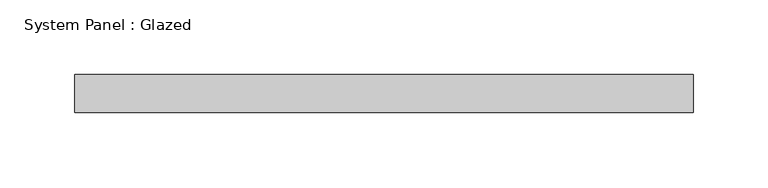
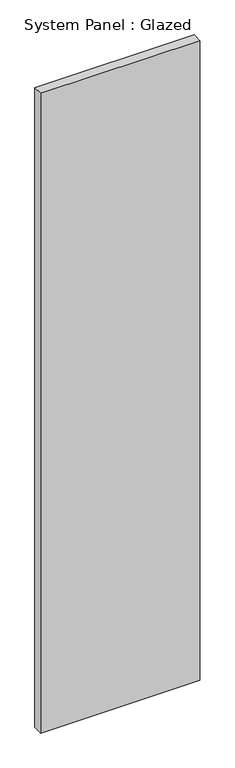
"""IFC4 building model written with IfcOpenShell, lengths in millimetres: plate geometry, System Panel : Glazed."""

from ifc_helpers import new_model, si_unit, origin, origin_with_axes, place, context, project, spatial, polyline, outline, extrude, source, transform, mapped, element, save


def system_panel_glazed_e2ad0beb(model_context):
    return source(origin(), model_context, "Body", "SweptSolid", [
        extrude(outline(polyline([(206.375, 19.05), (-206.375, 19.05), (-206.375, 44.45), (206.375, 44.45), (206.375, 19.05)])), origin_with_axes(), (0.0, 0.0, 1.0), 1752.6),
    ])


if __name__ == "__main__":
    model = new_model("IFC4")
    model_context = context("Model", 3, world=origin())
    ifc_project = project(units=[si_unit("LENGTHUNIT", "METRE", prefix="MILLI")], contexts=[model_context])
    site = spatial("IfcSite", under=ifc_project)
    building = spatial("IfcBuilding", under=site)
    placement = place(None, origin())
    system_panel_glazed_shape = system_panel_glazed_e2ad0beb(model_context)
    element("IfcPlate", 1, ObjectType="System Panel : Glazed", at=placement, inside=building, context=model_context, shape_type="MappedRepresentation", body=[
        mapped(system_panel_glazed_shape, transform((0.0, 0.0, 0.0), x_axis=(1.0, 0.0, 0.0), y_axis=(0.0, 1.0, 0.0), z_axis=(0.0, 0.0, 1.0))),
    ])
    save(model, "model.ifc")

# Revit data of these elements
# Type "System Panel : Glazed"
#   Construction Type Id = "GSP4R"
#   Analytic Construction = "1/8 in Pilkington single glazing"
#   Visual Light Transmittance = 0.9
#   Solar Heat Gain Coefficient = 0.86
#   Heat Transfer Coefficient (U) = 1.18115 BTU/(h·ft²·°F)
#   Define Thermal Properties by = 1
# Element 1 (IfcPlate, "System Panel : Glazed")
#   Materials on its faces: "Glass"
# Materials
#   "Glass": class "Glass", colour RGB 0 128 192, transparency 0.75, Description = "Soda Lime Glass", Cost = 0
